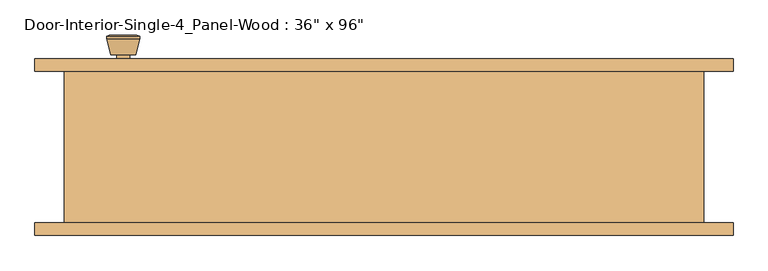
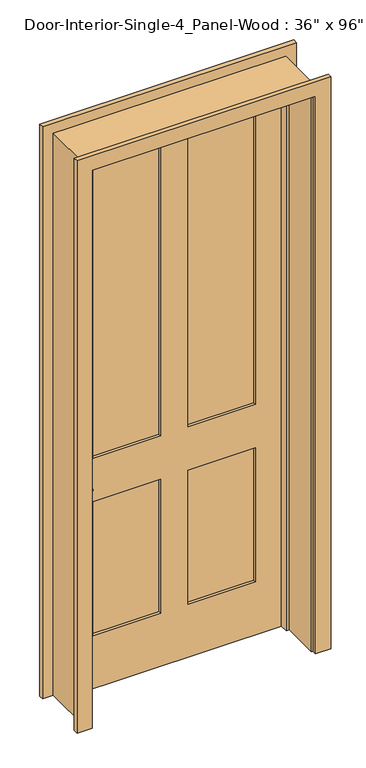
"""IFC4 building model written with IfcOpenShell, lengths in millimetres: door geometry."""

from ifc_helpers import new_model, si_unit, point, frame, frame_2d, origin, place, context, project, spatial, polyline, circle_curve, trimmed, segment, composite_curve, outline, extrude, faceted_brep, source, transform, mapped, element, save
from ifc_brep_helpers import plane_surface, cylinder_surface, revolved_surface, advanced_brep


def door_4f3f9908(model_context):
    return source(origin(), model_context, "Body", "SolidModel", [
        advanced_brep(
        [(-393.7, 70.2, 914.4), (-383.7, 70.2, 914.4), (-403.7, 70.2, 914.4), (-373.2241324, 21.2, 914.4), (-393.7, 21.2, 914.4), (-414.1758676, 21.2, 914.4), (-368.7, 23.0278681, 914.4), (-418.7, 23.0278681, 914.4), (-368.7, 26.4915463, 914.4), (-418.7, 26.4915463, 914.4), (-375.063764, 51.2, 914.4), (-412.336236, 51.2, 914.4), (-383.7, 51.2, 914.4), (-403.7, 51.2, 914.4)],
        [
            (0, 1),
            (1, 2, circle_curve(frame((-393.7, 70.2, 914.4), z_axis=(0.0, 1.0, 0.0), x_axis=(-1.0, 0.0, 0.0)), 10.0)),
            (2, 0),
            (2, 1, circle_curve(frame((-393.7, 70.2, 914.4), z_axis=(0.0, 1.0, 0.0), x_axis=(-1.0, 0.0, 0.0)), 10.0)),
            (3, 4),
            (4, 5),
            (5, 3, circle_curve(frame((-393.7, 21.2, 914.4), z_axis=(0.0, -1.0, 0.0), x_axis=(-1.0, 0.0, 0.0)), 20.4758676)),
            (3, 5, circle_curve(frame((-393.7, 21.2, 914.4), z_axis=(0.0, -1.0, 0.0), x_axis=(-1.0, 0.0, 0.0)), 20.4758676)),
            (6, 3),
            (5, 7),
            (7, 6, circle_curve(frame((-393.7, 23.0278681, 914.4), z_axis=(0.0, -1.0, 0.0), x_axis=(-1.0, 0.0, 0.0)), 25.0)),
            (6, 7, circle_curve(frame((-393.7, 23.0278681, 914.4), z_axis=(0.0, -1.0, 0.0), x_axis=(-1.0, 0.0, 0.0)), 25.0)),
            (8, 6),
            (7, 9),
            (9, 8, circle_curve(frame((-393.7, 26.4915463, 914.4), z_axis=(0.0, -1.0, 0.0), x_axis=(-1.0, 0.0, 0.0)), 25.0)),
            (8, 9, circle_curve(frame((-393.7, 26.4915463, 914.4), z_axis=(0.0, -1.0, 0.0), x_axis=(-1.0, 0.0, 0.0)), 25.0)),
            (10, 8),
            (9, 11),
            (11, 10, circle_curve(frame((-393.7, 51.2, 914.4), z_axis=(0.0, -1.0, 0.0), x_axis=(-1.0, 0.0, 0.0)), 18.636236)),
            (10, 11, circle_curve(frame((-393.7, 51.2, 914.4), z_axis=(0.0, -1.0, 0.0), x_axis=(-1.0, 0.0, 0.0)), 18.636236)),
            (12, 10),
            (11, 13),
            (13, 12, circle_curve(frame((-393.7, 51.2, 914.4), z_axis=(0.0, -1.0, 0.0), x_axis=(-1.0, 0.0, 0.0)), 10.0)),
            (12, 13, circle_curve(frame((-393.7, 51.2, 914.4), z_axis=(0.0, -1.0, 0.0), x_axis=(-1.0, 0.0, 0.0)), 10.0)),
            (1, 12),
            (13, 2),
        ],
        [
            plane_surface(frame((-393.7, 70.2, 914.4), z_axis=(0.0, 1.0, 0.0), x_axis=(-1.0, 0.0, 0.0))),
            plane_surface(frame((-393.7, 21.2, 914.4), z_axis=(0.0, -1.0, 0.0), x_axis=(-1.0, 0.0, 0.0))),
            revolved_surface(polyline([(-414.1758676, 21.2, 914.4), (-418.7, 23.0278681, 914.4)]), (-393.7, 70.2, 914.4), (0.0, 1.0, 0.0)),
            cylinder_surface(frame((-393.7, 70.2, 914.4), z_axis=(0.0, 1.0, 0.0), x_axis=(-1.0, 0.0, 0.0)), 25.0),
            revolved_surface(polyline([(-418.7, 26.4915463, 914.4), (-412.336236, 51.2, 914.4)]), (-393.7, 70.2, 914.4), (0.0, 1.0, 0.0)),
            plane_surface(frame((-393.7, 51.2, 914.4), z_axis=(0.0, 1.0, 0.0), x_axis=(-1.0, 0.0, 0.0))),
            cylinder_surface(frame((-393.7, 70.2, 914.4), z_axis=(0.0, 1.0, 0.0), x_axis=(-1.0, 0.0, 0.0)), 10.0),
        ],
        [
            (0, [[1, 2, 3]]),
            (0, [[-3, 4, -1]]),
            (1, [[5, 6, 7]]),
            (1, [[-6, -5, 8]]),
            (2, [[9, -7, 10, 11]]),
            (2, [[-10, -8, -9, 12]]),
            (3, [[13, -11, 14, 15]]),
            (3, [[-14, -12, -13, 16]]),
            (4, [[17, -15, 18, 19]]),
            (4, [[-18, -16, -17, 20]]),
            (5, [[21, -19, 22, 23]]),
            (5, [[-22, -20, -21, 24]]),
            (6, [[25, -23, 26, -2]]),
            (6, [[-26, -24, -25, -4]]),
        ],
    ),
        extrude(outline(composite_curve([segment(trimmed(circle_curve(frame_2d((914.4, -393.7)), 30.0), [point((914.4, -423.7))], [point((914.4, -363.7))], False, "CARTESIAN"), True, "CONTINUOUS"), segment(trimmed(circle_curve(frame_2d((914.4, -393.7)), 30.0), [point((914.4, -363.7))], [point((914.4, -423.7))], False, "CARTESIAN"), True, "CONTINUOUS")], self_intersect=False)), frame((0.0, 70.2, 0.0), z_axis=(0.0, 1.0, 0.0), x_axis=(0.0, 0.0, 1.0)), (0.0, 0.0, 1.0), 6.0),
        advanced_brep(
        [(-393.7, 117.125, 914.4), (-403.7, 117.125, 914.4), (-383.7, 117.125, 914.4), (-373.2241324, 166.125, 914.4), (-414.1758676, 166.125, 914.4), (-393.7, 166.125, 914.4), (-368.7, 164.2971319, 914.4), (-418.7, 164.2971319, 914.4), (-368.7, 160.8334537, 914.4), (-418.7, 160.8334537, 914.4), (-375.063764, 136.125, 914.4), (-412.336236, 136.125, 914.4), (-383.7, 136.125, 914.4), (-403.7, 136.125, 914.4)],
        [
            (0, 1),
            (1, 2, circle_curve(frame((-393.7, 117.125, 914.4), z_axis=(0.0, -1.0, 0.0), x_axis=(-1.0, 0.0, 0.0)), 10.0)),
            (2, 0),
            (2, 1, circle_curve(frame((-393.7, 117.125, 914.4), z_axis=(0.0, -1.0, 0.0), x_axis=(-1.0, 0.0, 0.0)), 10.0)),
            (3, 4, circle_curve(frame((-393.7, 166.125, 914.4), z_axis=(0.0, 1.0, 0.0), x_axis=(-1.0, 0.0, 0.0)), 20.4758676)),
            (4, 5),
            (5, 3),
            (4, 3, circle_curve(frame((-393.7, 166.125, 914.4), z_axis=(0.0, 1.0, 0.0), x_axis=(-1.0, 0.0, 0.0)), 20.4758676)),
            (6, 7, circle_curve(frame((-393.7, 164.2971319, 914.4), z_axis=(0.0, 1.0, 0.0), x_axis=(-1.0, 0.0, 0.0)), 25.0)),
            (7, 4),
            (3, 6),
            (7, 6, circle_curve(frame((-393.7, 164.2971319, 914.4), z_axis=(0.0, 1.0, 0.0), x_axis=(-1.0, 0.0, 0.0)), 25.0)),
            (8, 9, circle_curve(frame((-393.7, 160.8334537, 914.4), z_axis=(0.0, 1.0, 0.0), x_axis=(-1.0, 0.0, 0.0)), 25.0)),
            (9, 7),
            (6, 8),
            (9, 8, circle_curve(frame((-393.7, 160.8334537, 914.4), z_axis=(0.0, 1.0, 0.0), x_axis=(-1.0, 0.0, 0.0)), 25.0)),
            (10, 11, circle_curve(frame((-393.7, 136.125, 914.4), z_axis=(0.0, 1.0, 0.0), x_axis=(-1.0, 0.0, 0.0)), 18.636236)),
            (11, 9),
            (8, 10),
            (11, 10, circle_curve(frame((-393.7, 136.125, 914.4), z_axis=(0.0, 1.0, 0.0), x_axis=(-1.0, 0.0, 0.0)), 18.636236)),
            (12, 13, circle_curve(frame((-393.7, 136.125, 914.4), z_axis=(0.0, 1.0, 0.0), x_axis=(-1.0, 0.0, 0.0)), 10.0)),
            (13, 11),
            (10, 12),
            (13, 12, circle_curve(frame((-393.7, 136.125, 914.4), z_axis=(0.0, 1.0, 0.0), x_axis=(-1.0, 0.0, 0.0)), 10.0)),
            (1, 13),
            (12, 2),
        ],
        [
            plane_surface(frame((-393.7, 117.125, 914.4), z_axis=(0.0, -1.0, 0.0), x_axis=(-1.0, 0.0, 0.0))),
            plane_surface(frame((-393.7, 166.125, 914.4), z_axis=(0.0, 1.0, 0.0), x_axis=(-1.0, 0.0, 0.0))),
            revolved_surface(polyline([(-414.1758676, 166.125, 914.4), (-418.7, 164.2971319, 914.4)]), (-393.7, 117.125, 914.4), (0.0, -1.0, 0.0)),
            cylinder_surface(frame((-393.7, 117.125, 914.4), z_axis=(0.0, -1.0, 0.0), x_axis=(-1.0, 0.0, 0.0)), 25.0),
            revolved_surface(polyline([(-418.7, 160.8334537, 914.4), (-412.336236, 136.125, 914.4)]), (-393.7, 117.125, 914.4), (0.0, -1.0, 0.0)),
            plane_surface(frame((-393.7, 136.125, 914.4), z_axis=(0.0, -1.0, 0.0), x_axis=(-1.0, 0.0, 0.0))),
            cylinder_surface(frame((-393.7, 117.125, 914.4), z_axis=(0.0, -1.0, 0.0), x_axis=(-1.0, 0.0, 0.0)), 10.0),
        ],
        [
            (0, [[1, 2, 3]]),
            (0, [[-3, 4, -1]]),
            (1, [[5, 6, 7]]),
            (1, [[8, -7, -6]]),
            (2, [[9, 10, -5, 11]]),
            (2, [[12, -11, -8, -10]]),
            (3, [[13, 14, -9, 15]]),
            (3, [[16, -15, -12, -14]]),
            (4, [[17, 18, -13, 19]]),
            (4, [[20, -19, -16, -18]]),
            (5, [[21, 22, -17, 23]]),
            (5, [[24, -23, -20, -22]]),
            (6, [[-2, 25, -21, 26]]),
            (6, [[-4, -26, -24, -25]]),
        ],
    ),
        extrude(outline(composite_curve([segment(trimmed(circle_curve(frame_2d((914.4, -393.7)), 30.0), [point((914.4, -423.7))], [point((914.4, -363.7))], False, "CARTESIAN"), True, "CONTINUOUS"), segment(trimmed(circle_curve(frame_2d((914.4, -393.7)), 30.0), [point((914.4, -363.7))], [point((914.4, -423.7))], False, "CARTESIAN"), True, "CONTINUOUS")], self_intersect=False)), frame((0.0, 111.125, 0.0), z_axis=(0.0, 1.0, 0.0), x_axis=(0.0, 0.0, 1.0)), (0.0, 0.0, 1.0), 6.0),
        faceted_brep([(482.6, 111.125, 0.0), (482.6, -117.475, 0.0), (457.2, -117.475, 0.0), (457.2, 41.275, 0.0), (444.5, 41.275, 0.0), (444.5, 76.2, 0.0), (457.2, 76.2, 0.0), (457.2, 111.125, 0.0), (482.6, 111.125, 2463.8), (482.6, -117.475, 2463.8), (-482.6, -117.475, 2463.8), (-482.6, -117.475, 0.0), (-457.2, -117.475, 0.0), (-457.2, -117.475, 2438.4), (457.2, -117.475, 2438.4), (457.2, 41.275, 2438.4), (-457.2, 41.275, 2438.4), (-457.2, 41.275, 0.0), (-444.5, 41.275, 0.0), (-444.5, 41.275, 2425.7), (444.5, 41.275, 2425.7), (444.5, 76.2, 2425.7), (-444.5, 76.2, 2425.7), (-444.5, 76.2, 0.0), (-457.2, 76.2, 0.0), (-457.2, 76.2, 2438.4), (457.2, 76.2, 2438.4), (457.2, 111.125, 2438.4), (-457.2, 111.125, 2438.4), (-457.2, 111.125, 0.0), (-482.6, 111.125, 0.0), (-482.6, 111.125, 2463.8)], [[[0, 1, 2, 3, 4, 5, 6, 7]], [[1, 0, 8, 9]], [[2, 1, 9, 10, 11, 12, 13, 14]], [[3, 2, 14, 15]], [[4, 3, 15, 16, 17, 18, 19, 20]], [[5, 4, 20, 21]], [[6, 5, 21, 22, 23, 24, 25, 26]], [[7, 6, 26, 27]], [[0, 7, 27, 28, 29, 30, 31, 8]], [[9, 8, 31, 10]], [[15, 14, 13, 16]], [[21, 20, 19, 22]], [[27, 26, 25, 28]], [[30, 29, 24, 23, 18, 17, 12, 11]], [[10, 31, 30, 11]], [[16, 13, 12, 17]], [[22, 19, 18, 23]], [[28, 25, 24, 29]]]),
        extrude(outline(polyline([(2438.4, -457.2), (0.0, -457.2), (0.0, 457.2), (2438.4, 457.2), (2438.4, -457.2)]), holes=[polyline([(2319.3375, 57.15), (2319.3375, 336.55), (1009.65, 336.55), (1009.65, 57.15), (2319.3375, 57.15)]), polyline([(1009.65, -57.15), (1009.65, -336.55), (2319.3375, -336.55), (2319.3375, -57.15), (1009.65, -57.15)]), polyline([(819.15, 57.15), (819.15, 336.55), (231.775, 336.55), (231.775, 57.15), (819.15, 57.15)]), polyline([(231.775, -57.15), (231.775, -336.55), (819.15, -336.55), (819.15, -57.15), (231.775, -57.15)])]), frame((0.0, 76.2, 0.0), z_axis=(0.0, 1.0, 0.0), x_axis=(0.0, 0.0, 1.0)), (0.0, 0.0, 1.0), 34.925),
        extrude(outline(polyline([(336.55, 87.8416667), (57.15, 87.8416667), (57.15, 99.4833333), (336.55, 99.4833333), (336.55, 87.8416667)])), frame((0.0, 0.0, 1009.65), z_axis=(0.0, 0.0, 1.0), x_axis=(1.0, 0.0, 0.0)), (0.0, 0.0, 1.0), 1309.6875),
        extrude(outline(polyline([(-57.15, 87.8416667), (-336.55, 87.8416667), (-336.55, 99.4833333), (-57.15, 99.4833333), (-57.15, 87.8416667)])), frame((0.0, 0.0, 1009.65), z_axis=(0.0, 0.0, 1.0), x_axis=(1.0, 0.0, 0.0)), (0.0, 0.0, 1.0), 1309.6875),
        extrude(outline(polyline([(336.55, 87.8416667), (57.15, 87.8416667), (57.15, 99.4833333), (336.55, 99.4833333), (336.55, 87.8416667)])), frame((0.0, 0.0, 231.775), z_axis=(0.0, 0.0, 1.0), x_axis=(1.0, 0.0, 0.0)), (0.0, 0.0, 1.0), 587.375),
        extrude(outline(polyline([(-57.15, 87.8416667), (-336.55, 87.8416667), (-336.55, 99.4833333), (-57.15, 99.4833333), (-57.15, 87.8416667)])), frame((0.0, 0.0, 231.775), z_axis=(0.0, 0.0, 1.0), x_axis=(1.0, 0.0, 0.0)), (0.0, 0.0, 1.0), 587.375),
        extrude(outline(polyline([(0.0, 463.55), (0.0, 527.05), (2508.25, 527.05), (2508.25, -527.05), (0.0, -527.05), (0.0, -463.55), (2444.75, -463.55), (2444.75, 463.55), (0.0, 463.55)])), frame((0.0, 111.125, 0.0), z_axis=(0.0, 1.0, 0.0), x_axis=(0.0, 0.0, 1.0)), (0.0, 0.0, 1.0), 19.05),
        extrude(outline(polyline([(0.0, 463.55), (0.0, 527.05), (2508.25, 527.05), (2508.25, -527.05), (0.0, -527.05), (0.0, -463.55), (2444.75, -463.55), (2444.75, 463.55), (0.0, 463.55)])), frame((0.0, -136.525, 0.0), z_axis=(0.0, 1.0, 0.0), x_axis=(0.0, 0.0, 1.0)), (0.0, 0.0, 1.0), 19.05),
    ])


if __name__ == "__main__":
    model = new_model("IFC4")
    model_context = context("Model", 3, world=origin())
    ifc_project = project(units=[si_unit("LENGTHUNIT", "METRE", prefix="MILLI")], contexts=[model_context])
    site = spatial("IfcSite", under=ifc_project)
    building = spatial("IfcBuilding", under=site)
    placement = place(None, origin())
    door_shape = door_4f3f9908(model_context)
    element("IfcDoor", 1, ObjectType="Door-Interior-Single-4_Panel-Wood : 36\" x 96\"", at=placement, inside=building, context=model_context, shape_type="MappedRepresentation", body=[
        mapped(door_shape, transform((0.0, 0.0, 0.0), x_axis=(1.0, 0.0, 0.0), y_axis=(0.0, 1.0, 0.0), z_axis=(0.0, 0.0, 1.0))),
    ])
    save(model, "model.ifc")

# Revit data of these elements
# Type "Door-Interior-Single-4_Panel-Wood : 36\" x 96\""
#   Type Mark = "9"
#   Assembly Code = "C1020300"
#   Analytic Construction = "Wooden"
#   Top Rail = 0' - 4 11/16"
#   Thickness = 0' - 1 3/8"
#   Thermal Resistance (R) = 2.5876 (h·ft²·°F)/BTU
#   Swing Angle [instance default] = 90.00°
#   Stiles = 0' - 4 3/4"
#   Rough Width = 3' - 2"
#   Rough Height = 8' - 1"
#   Mullion = 0' - 4 1/2"
#   Lock Rail = 0' - 7 1/2"
#   Height = 8' - 0"
#   Width = 3' - 0"
#   Heat Transfer Coefficient (U) = 0.3865 BTU/(h·ft²·°F)
#   Bottom Rail = 0' - 9 1/8"
#   Trim Material = Cherry
#   Panel Material = Cherry
#   Frame Material = Cherry
#   Door Handle Material = Aluminum
#   Visual Light Transmittance = 0
#   Solar Heat Gain Coefficient = 0
#   Wall Closure = (empty or 0)
#   Function = (empty or 0)
# Element 1 (IfcDoor, "Door-Interior-Single-4_Panel-Wood : 36\" x 96\"")
#   Materials on its faces: "Cherry", "Aluminum"
# Materials
#   "Cherry": class "Wood", colour RGB 226 177 128, transparency 0, Description = "Prunus Serotina", Cost = 0
#   "Aluminum": class "Metal", colour RGB 247 247 247, transparency 0, Description = "Aluminum 6061", Cost = 0
